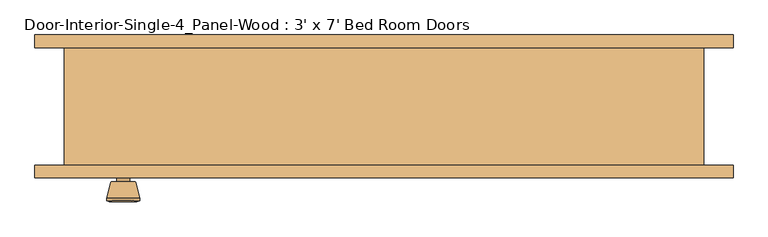
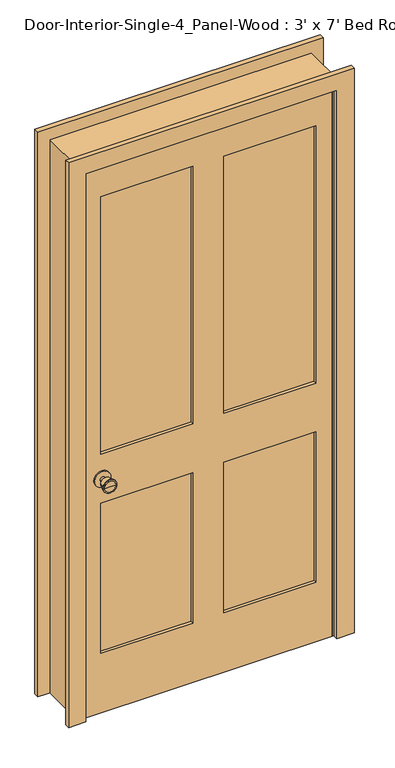
"""IFC4 building model written with IfcOpenShell, lengths in millimetres: door geometry, Door-Interior-Single-4_Panel-Wood : 3' x 7' Bed Room Doors."""

from ifc_helpers import new_model, si_unit, point, frame, frame_2d, origin, place, context, project, spatial, polyline, circle_curve, trimmed, segment, composite_curve, outline, extrude, faceted_brep, source, transform, mapped, element, save
from ifc_brep_helpers import plane_surface, cylinder_surface, revolved_surface, advanced_brep


def door_interior_single_4_panel_wood_3_x_7_bed_room_doors_167030f9(model_context):
    return source(origin(), model_context, "Body", "SolidModel", [
        advanced_brep(
        [(-393.7, -44.8, 914.4), (-403.7, -44.8, 914.4), (-383.7, -44.8, 914.4), (-373.2241324, 4.2, 914.4), (-414.1758676, 4.2, 914.4), (-393.7, 4.2, 914.4), (-368.7, 2.3721319, 914.4), (-418.7, 2.3721319, 914.4), (-368.7, -1.0915463, 914.4), (-418.7, -1.0915463, 914.4), (-375.063764, -25.8, 914.4), (-412.336236, -25.8, 914.4), (-383.7, -25.8, 914.4), (-403.7, -25.8, 914.4)],
        [
            (0, 1),
            (1, 2, circle_curve(frame((-393.7, -44.8, 914.4), z_axis=(0.0, -1.0, 0.0), x_axis=(-1.0, 0.0, 0.0)), 10.0)),
            (2, 0),
            (2, 1, circle_curve(frame((-393.7, -44.8, 914.4), z_axis=(0.0, -1.0, 0.0), x_axis=(-1.0, 0.0, 0.0)), 10.0)),
            (3, 4, circle_curve(frame((-393.7, 4.2, 914.4), z_axis=(0.0, 1.0, 0.0), x_axis=(-1.0, 0.0, 0.0)), 20.4758676)),
            (4, 5),
            (5, 3),
            (4, 3, circle_curve(frame((-393.7, 4.2, 914.4), z_axis=(0.0, 1.0, 0.0), x_axis=(-1.0, 0.0, 0.0)), 20.4758676)),
            (6, 7, circle_curve(frame((-393.7, 2.3721319, 914.4), z_axis=(0.0, 1.0, 0.0), x_axis=(-1.0, 0.0, 0.0)), 25.0)),
            (7, 4),
            (3, 6),
            (7, 6, circle_curve(frame((-393.7, 2.3721319, 914.4), z_axis=(0.0, 1.0, 0.0), x_axis=(-1.0, 0.0, 0.0)), 25.0)),
            (8, 9, circle_curve(frame((-393.7, -1.0915463, 914.4), z_axis=(0.0, 1.0, 0.0), x_axis=(-1.0, 0.0, 0.0)), 25.0)),
            (9, 7),
            (6, 8),
            (9, 8, circle_curve(frame((-393.7, -1.0915463, 914.4), z_axis=(0.0, 1.0, 0.0), x_axis=(-1.0, 0.0, 0.0)), 25.0)),
            (10, 11, circle_curve(frame((-393.7, -25.8, 914.4), z_axis=(0.0, 1.0, 0.0), x_axis=(-1.0, 0.0, 0.0)), 18.636236)),
            (11, 9),
            (8, 10),
            (11, 10, circle_curve(frame((-393.7, -25.8, 914.4), z_axis=(0.0, 1.0, 0.0), x_axis=(-1.0, 0.0, 0.0)), 18.636236)),
            (12, 13, circle_curve(frame((-393.7, -25.8, 914.4), z_axis=(0.0, 1.0, 0.0), x_axis=(-1.0, 0.0, 0.0)), 10.0)),
            (13, 11),
            (10, 12),
            (13, 12, circle_curve(frame((-393.7, -25.8, 914.4), z_axis=(0.0, 1.0, 0.0), x_axis=(-1.0, 0.0, 0.0)), 10.0)),
            (1, 13),
            (12, 2),
        ],
        [
            plane_surface(frame((-393.7, -44.8, 914.4), z_axis=(0.0, -1.0, 0.0), x_axis=(-1.0, 0.0, 0.0))),
            plane_surface(frame((-393.7, 4.2, 914.4), z_axis=(0.0, 1.0, 0.0), x_axis=(-1.0, 0.0, 0.0))),
            revolved_surface(polyline([(-414.1758676, 4.2, 914.4), (-418.7, 2.3721319, 914.4)]), (-393.7, -44.8, 914.4), (0.0, -1.0, 0.0)),
            cylinder_surface(frame((-393.7, -44.8, 914.4), z_axis=(0.0, -1.0, 0.0), x_axis=(-1.0, 0.0, 0.0)), 25.0),
            revolved_surface(polyline([(-418.7, -1.0915463, 914.4), (-412.336236, -25.8, 914.4)]), (-393.7, -44.8, 914.4), (0.0, -1.0, 0.0)),
            plane_surface(frame((-393.7, -25.8, 914.4), z_axis=(0.0, -1.0, 0.0), x_axis=(-1.0, 0.0, 0.0))),
            cylinder_surface(frame((-393.7, -44.8, 914.4), z_axis=(0.0, -1.0, 0.0), x_axis=(-1.0, 0.0, 0.0)), 10.0),
        ],
        [
            (0, [[1, 2, 3]]),
            (0, [[-3, 4, -1]]),
            (1, [[5, 6, 7]]),
            (1, [[8, -7, -6]]),
            (2, [[9, 10, -5, 11]]),
            (2, [[12, -11, -8, -10]]),
            (3, [[13, 14, -9, 15]]),
            (3, [[16, -15, -12, -14]]),
            (4, [[17, 18, -13, 19]]),
            (4, [[20, -19, -16, -18]]),
            (5, [[21, 22, -17, 23]]),
            (5, [[24, -23, -20, -22]]),
            (6, [[-2, 25, -21, 26]]),
            (6, [[-4, -26, -24, -25]]),
        ],
    ),
        extrude(outline(composite_curve([segment(trimmed(circle_curve(frame_2d((914.4, -393.7)), 30.0), [point((914.4, -423.7))], [point((914.4, -363.7))], False, "CARTESIAN"), True, "CONTINUOUS"), segment(trimmed(circle_curve(frame_2d((914.4, -393.7)), 30.0), [point((914.4, -363.7))], [point((914.4, -423.7))], False, "CARTESIAN"), True, "CONTINUOUS")], self_intersect=False)), frame((0.0, -50.8, 0.0), z_axis=(0.0, 1.0, 0.0), x_axis=(0.0, 0.0, 1.0)), (0.0, 0.0, 1.0), 6.0),
        advanced_brep(
        [(-393.7, -91.725, 914.4), (-383.7, -91.725, 914.4), (-403.7, -91.725, 914.4), (-373.2241324, -140.725, 914.4), (-393.7, -140.725, 914.4), (-414.1758676, -140.725, 914.4), (-368.7, -138.8971319, 914.4), (-418.7, -138.8971319, 914.4), (-368.7, -135.4334537, 914.4), (-418.7, -135.4334537, 914.4), (-375.063764, -110.725, 914.4), (-412.336236, -110.725, 914.4), (-383.7, -110.725, 914.4), (-403.7, -110.725, 914.4)],
        [
            (0, 1),
            (1, 2, circle_curve(frame((-393.7, -91.725, 914.4), z_axis=(0.0, 1.0, 0.0), x_axis=(-1.0, 0.0, 0.0)), 10.0)),
            (2, 0),
            (2, 1, circle_curve(frame((-393.7, -91.725, 914.4), z_axis=(0.0, 1.0, 0.0), x_axis=(-1.0, 0.0, 0.0)), 10.0)),
            (3, 4),
            (4, 5),
            (5, 3, circle_curve(frame((-393.7, -140.725, 914.4), z_axis=(0.0, -1.0, 0.0), x_axis=(-1.0, 0.0, 0.0)), 20.4758676)),
            (3, 5, circle_curve(frame((-393.7, -140.725, 914.4), z_axis=(0.0, -1.0, 0.0), x_axis=(-1.0, 0.0, 0.0)), 20.4758676)),
            (6, 3),
            (5, 7),
            (7, 6, circle_curve(frame((-393.7, -138.8971319, 914.4), z_axis=(0.0, -1.0, 0.0), x_axis=(-1.0, 0.0, 0.0)), 25.0)),
            (6, 7, circle_curve(frame((-393.7, -138.8971319, 914.4), z_axis=(0.0, -1.0, 0.0), x_axis=(-1.0, 0.0, 0.0)), 25.0)),
            (8, 6),
            (7, 9),
            (9, 8, circle_curve(frame((-393.7, -135.4334537, 914.4), z_axis=(0.0, -1.0, 0.0), x_axis=(-1.0, 0.0, 0.0)), 25.0)),
            (8, 9, circle_curve(frame((-393.7, -135.4334537, 914.4), z_axis=(0.0, -1.0, 0.0), x_axis=(-1.0, 0.0, 0.0)), 25.0)),
            (10, 8),
            (9, 11),
            (11, 10, circle_curve(frame((-393.7, -110.725, 914.4), z_axis=(0.0, -1.0, 0.0), x_axis=(-1.0, 0.0, 0.0)), 18.636236)),
            (10, 11, circle_curve(frame((-393.7, -110.725, 914.4), z_axis=(0.0, -1.0, 0.0), x_axis=(-1.0, 0.0, 0.0)), 18.636236)),
            (12, 10),
            (11, 13),
            (13, 12, circle_curve(frame((-393.7, -110.725, 914.4), z_axis=(0.0, -1.0, 0.0), x_axis=(-1.0, 0.0, 0.0)), 10.0)),
            (12, 13, circle_curve(frame((-393.7, -110.725, 914.4), z_axis=(0.0, -1.0, 0.0), x_axis=(-1.0, 0.0, 0.0)), 10.0)),
            (1, 12),
            (13, 2),
        ],
        [
            plane_surface(frame((-393.7, -91.725, 914.4), z_axis=(0.0, 1.0, 0.0), x_axis=(-1.0, 0.0, 0.0))),
            plane_surface(frame((-393.7, -140.725, 914.4), z_axis=(0.0, -1.0, 0.0), x_axis=(-1.0, 0.0, 0.0))),
            revolved_surface(polyline([(-414.1758676, -140.725, 914.4), (-418.7, -138.8971319, 914.4)]), (-393.7, -91.725, 914.4), (0.0, 1.0, 0.0)),
            cylinder_surface(frame((-393.7, -91.725, 914.4), z_axis=(0.0, 1.0, 0.0), x_axis=(-1.0, 0.0, 0.0)), 25.0),
            revolved_surface(polyline([(-418.7, -135.4334537, 914.4), (-412.336236, -110.725, 914.4)]), (-393.7, -91.725, 914.4), (0.0, 1.0, 0.0)),
            plane_surface(frame((-393.7, -110.725, 914.4), z_axis=(0.0, 1.0, 0.0), x_axis=(-1.0, 0.0, 0.0))),
            cylinder_surface(frame((-393.7, -91.725, 914.4), z_axis=(0.0, 1.0, 0.0), x_axis=(-1.0, 0.0, 0.0)), 10.0),
        ],
        [
            (0, [[1, 2, 3]]),
            (0, [[-3, 4, -1]]),
            (1, [[5, 6, 7]]),
            (1, [[-6, -5, 8]]),
            (2, [[9, -7, 10, 11]]),
            (2, [[-10, -8, -9, 12]]),
            (3, [[13, -11, 14, 15]]),
            (3, [[-14, -12, -13, 16]]),
            (4, [[17, -15, 18, 19]]),
            (4, [[-18, -16, -17, 20]]),
            (5, [[21, -19, 22, 23]]),
            (5, [[-22, -20, -21, 24]]),
            (6, [[25, -23, 26, -2]]),
            (6, [[-26, -24, -25, -4]]),
        ],
    ),
        extrude(outline(composite_curve([segment(trimmed(circle_curve(frame_2d((914.4, -393.7)), 30.0), [point((914.4, -423.7))], [point((914.4, -363.7))], False, "CARTESIAN"), True, "CONTINUOUS"), segment(trimmed(circle_curve(frame_2d((914.4, -393.7)), 30.0), [point((914.4, -363.7))], [point((914.4, -423.7))], False, "CARTESIAN"), True, "CONTINUOUS")], self_intersect=False)), frame((0.0, -91.725, 0.0), z_axis=(0.0, 1.0, 0.0), x_axis=(0.0, 0.0, 1.0)), (0.0, 0.0, 1.0), 6.0),
        faceted_brep([(482.6, -85.725, 0.0), (457.2, -85.725, 0.0), (457.2, -50.8, 0.0), (444.5, -50.8, 0.0), (444.5, -15.875, 0.0), (457.2, -15.875, 0.0), (457.2, 92.075, 0.0), (482.6, 92.075, 0.0), (482.6, 92.075, 2159.0), (482.6, -85.725, 2159.0), (457.2, 92.075, 2133.6), (-457.2, 92.075, 2133.6), (-457.2, 92.075, 0.0), (-482.6, 92.075, 0.0), (-482.6, 92.075, 2159.0), (457.2, -15.875, 2133.6), (444.5, -15.875, 2120.9), (-444.5, -15.875, 2120.9), (-444.5, -15.875, 0.0), (-457.2, -15.875, 0.0), (-457.2, -15.875, 2133.6), (444.5, -50.8, 2120.9), (457.2, -50.8, 2133.6), (-457.2, -50.8, 2133.6), (-457.2, -50.8, 0.0), (-444.5, -50.8, 0.0), (-444.5, -50.8, 2120.9), (457.2, -85.725, 2133.6), (-482.6, -85.725, 2159.0), (-482.6, -85.725, 0.0), (-457.2, -85.725, 0.0), (-457.2, -85.725, 2133.6)], [[[0, 1, 2, 3, 4, 5, 6, 7]], [[7, 8, 9, 0]], [[6, 10, 11, 12, 13, 14, 8, 7]], [[5, 15, 10, 6]], [[4, 16, 17, 18, 19, 20, 15, 5]], [[3, 21, 16, 4]], [[2, 22, 23, 24, 25, 26, 21, 3]], [[1, 27, 22, 2]], [[0, 9, 28, 29, 30, 31, 27, 1]], [[8, 14, 28, 9]], [[15, 20, 11, 10]], [[21, 26, 17, 16]], [[27, 31, 23, 22]], [[29, 13, 12, 19, 18, 25, 24, 30]], [[14, 13, 29, 28]], [[20, 19, 12, 11]], [[26, 25, 18, 17]], [[31, 30, 24, 23]]]),
        extrude(outline(polyline([(2133.6, -457.2), (0.0, -457.2), (0.0, 457.2), (2133.6, 457.2), (2133.6, -457.2)]), holes=[polyline([(2014.5375, 57.15), (2014.5375, 396.875), (1009.65, 396.875), (1009.65, 57.15), (2014.5375, 57.15)]), polyline([(1009.65, -57.15), (1009.65, -396.875), (2014.5375, -396.875), (2014.5375, -57.15), (1009.65, -57.15)]), polyline([(819.15, 57.15), (819.15, 396.875), (231.775, 396.875), (231.775, 57.15), (819.15, 57.15)]), polyline([(231.775, -57.15), (231.775, -396.875), (819.15, -396.875), (819.15, -57.15), (231.775, -57.15)])]), frame((0.0, -85.725, 0.0), z_axis=(0.0, 1.0, 0.0), x_axis=(0.0, 0.0, 1.0)), (0.0, 0.0, 1.0), 34.925),
        extrude(outline(polyline([(396.875, -62.4416667), (396.875, -74.0833333), (57.15, -74.0833333), (57.15, -62.4416667), (396.875, -62.4416667)])), frame((0.0, 0.0, 1009.65), z_axis=(0.0, 0.0, 1.0), x_axis=(1.0, 0.0, 0.0)), (0.0, 0.0, 1.0), 1004.8875),
        extrude(outline(polyline([(-57.15, -62.4416667), (-57.15, -74.0833333), (-396.875, -74.0833333), (-396.875, -62.4416667), (-57.15, -62.4416667)])), frame((0.0, 0.0, 1009.65), z_axis=(0.0, 0.0, 1.0), x_axis=(1.0, 0.0, 0.0)), (0.0, 0.0, 1.0), 1004.8875),
        extrude(outline(polyline([(396.875, -62.4416667), (396.875, -74.0833333), (57.15, -74.0833333), (57.15, -62.4416667), (396.875, -62.4416667)])), frame((0.0, 0.0, 231.775), z_axis=(0.0, 0.0, 1.0), x_axis=(1.0, 0.0, 0.0)), (0.0, 0.0, 1.0), 587.375),
        extrude(outline(polyline([(-57.15, -62.4416667), (-57.15, -74.0833333), (-396.875, -74.0833333), (-396.875, -62.4416667), (-57.15, -62.4416667)])), frame((0.0, 0.0, 231.775), z_axis=(0.0, 0.0, 1.0), x_axis=(1.0, 0.0, 0.0)), (0.0, 0.0, 1.0), 587.375),
        extrude(outline(polyline([(0.0, 527.05), (2203.45, 527.05), (2203.45, -527.05), (0.0, -527.05), (0.0, -463.55), (2139.95, -463.55), (2139.95, 463.55), (0.0, 463.55), (0.0, 527.05)])), frame((0.0, -104.775, 0.0), z_axis=(0.0, 1.0, 0.0), x_axis=(0.0, 0.0, 1.0)), (0.0, 0.0, 1.0), 19.05),
        extrude(outline(polyline([(0.0, 527.05), (2203.45, 527.05), (2203.45, -527.05), (0.0, -527.05), (0.0, -463.55), (2139.95, -463.55), (2139.95, 463.55), (0.0, 463.55), (0.0, 527.05)])), frame((0.0, 92.075, 0.0), z_axis=(0.0, 1.0, 0.0), x_axis=(0.0, 0.0, 1.0)), (0.0, 0.0, 1.0), 19.05),
    ])


if __name__ == "__main__":
    model = new_model("IFC4")
    model_context = context("Model", 3, world=origin())
    ifc_project = project(units=[si_unit("LENGTHUNIT", "METRE", prefix="MILLI")], contexts=[model_context])
    site = spatial("IfcSite", under=ifc_project)
    building = spatial("IfcBuilding", under=site)
    placement = place(None, origin())
    door_interior_single_4_panel_wood_3_x_7_bed_room_doors_shape = door_interior_single_4_panel_wood_3_x_7_bed_room_doors_167030f9(model_context)
    element("IfcDoor", 1, ObjectType="Door-Interior-Single-4_Panel-Wood : 3' x 7' Bed Room Doors", at=placement, inside=building, context=model_context, shape_type="MappedRepresentation", body=[
        mapped(door_interior_single_4_panel_wood_3_x_7_bed_room_doors_shape, transform((0.0, 0.0, 0.0), x_axis=(1.0, 0.0, 0.0), y_axis=(0.0, 1.0, 0.0), z_axis=(0.0, 0.0, 1.0))),
    ])
    save(model, "model.ifc")

# Revit data of these elements
# Type "Door-Interior-Single-4_Panel-Wood : 3' x 7' Bed Room Doors"
#   Type Mark = "13"
#   Assembly Code = "C1020300"
#   Analytic Construction = "Wooden"
#   Top Rail = 0' - 4 11/16"
#   Thickness = 0' - 1 3/8"
#   Thermal Resistance (R) = 2.5876 (h·ft²·°F)/BTU
#   Swing Angle [instance default] = 90.00°
#   Stiles = 0' - 2 3/8"
#   Rough Width = 3' - 2"
#   Rough Height = 7' - 1"
#   Mullion = 0' - 4 1/2"
#   Lock Rail = 0' - 7 1/2"
#   Height = 7' - 0"
#   Width = 3' - 0"
#   Heat Transfer Coefficient (U) = 0.3865 BTU/(h·ft²·°F)
#   Bottom Rail = 0' - 9 1/8"
#   Trim Material = Cherry
#   Panel Material = Cherry
#   Frame Material = Cherry
#   Door Handle Material = Aluminum
#   Visual Light Transmittance = 0
#   Solar Heat Gain Coefficient = 0
#   Wall Closure = (empty or 0)
#   Function = (empty or 0)
# Element 1 (IfcDoor, "Door-Interior-Single-4_Panel-Wood : 3' x 7' Bed Room Doors")
#   Materials on its faces: "Cherry", "Aluminum"
# Materials
#   "Cherry": class "Wood", colour RGB 226 177 128, transparency 0, Description = "Prunus Serotina", Cost = 0
#   "Aluminum": class "Metal", colour RGB 247 247 247, transparency 0, Description = "Aluminum 6061", Cost = 0
